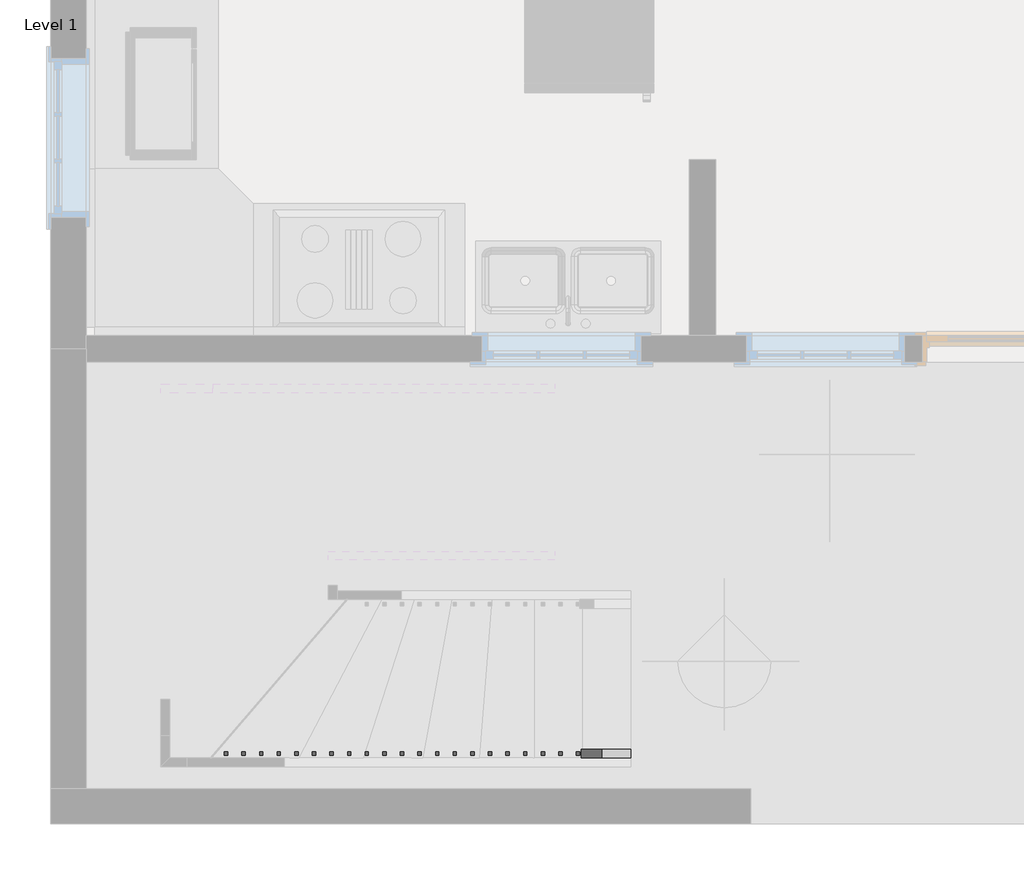
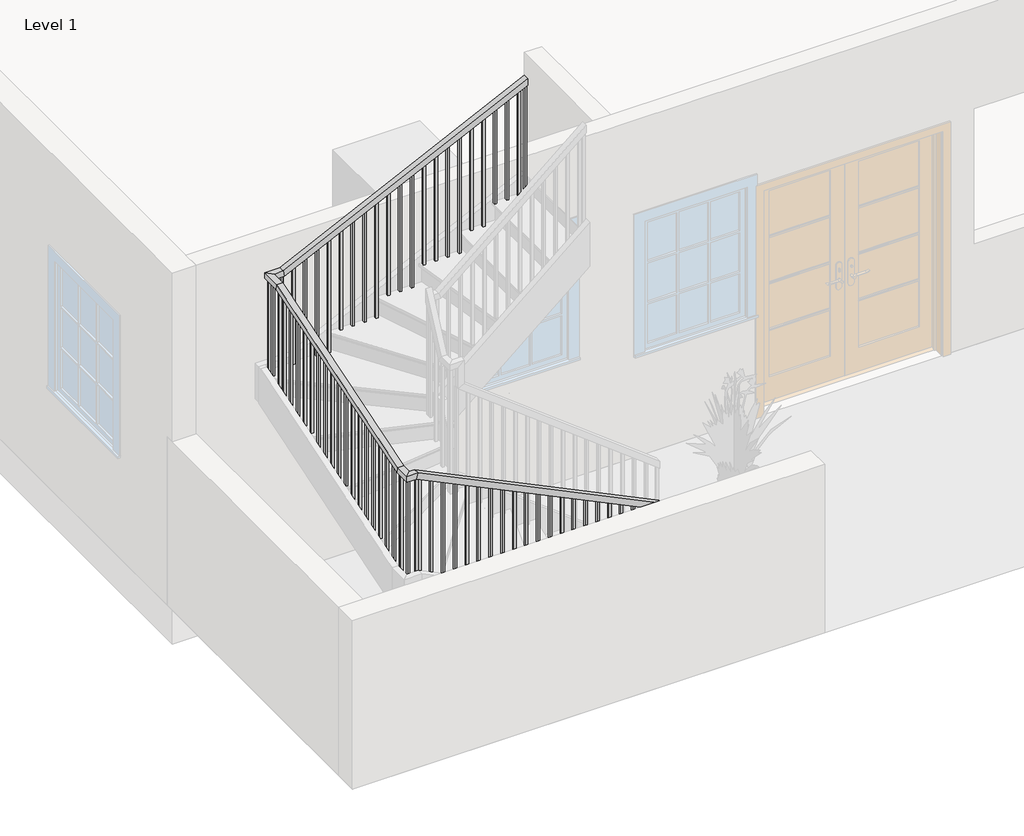
# One storey, part 2 of 3: 1 railing.
"""IFC4 building model written with IfcOpenShell, lengths in millimetres."""

from ifc_helpers import new_model, si_unit, frame, origin, place, context, project, spatial, polyline, outline, extrude, faceted_brep, element, save

model = new_model("IFC4")

# Units and contexts
model_context = context("Model", 3, world=origin())
ifc_project = project(units=[si_unit("LENGTHUNIT", "METRE", prefix="MILLI")], contexts=[model_context])

# Site, building, storey
site = spatial("IfcSite", under=ifc_project)
building = spatial("IfcBuilding", under=site)
storey = spatial("IfcBuildingStorey", under=building, Name="Level 1", Elevation=0.0)

# Railing
placement = place(None, origin())
element("IfcRailing", 1, ObjectType="Handrail - Rectangular", at=placement, inside=storey, context=model_context, shape_type="SolidModel", body=[
    faceted_brep([(-8086.227471, 2208.1174997, 1118.3371319), (-8086.227471, 2208.1174997, 1061.9393688), (-8086.227471, 2258.9174997, 1061.9393688), (-8086.227471, 2258.9174997, 1118.3371319), (-10651.2149162, 2208.1174997, 2355.2002855), (-10662.8234698, 2208.1174997, 2304.4002855), (-10662.8234698, 2258.9174997, 2304.4002855), (-10651.2149162, 2258.9174997, 2355.2002855), (-10747.2073372, 2208.1174997, 2355.2002855), (-10747.2073372, 2208.1174997, 2304.4002855), (-10696.4073372, 2258.9174997, 2304.4002855), (-10696.4073372, 2258.9174997, 2355.2002855), (-10747.2073372, 2341.0593041, 2355.2002855), (-10747.2073372, 2348.9073224, 2304.4002855), (-10696.4073372, 2348.9073224, 2304.4002855), (-10696.4073372, 2341.0593041, 2355.2002855), (-10747.2073372, 4134.1159277, 2922.7594886), (-10747.2073372, 4141.963946, 2871.9594886), (-10696.4073372, 4141.963946, 2871.9594886), (-10696.4073372, 4134.1159277, 2922.7594886), (-10747.2073372, 4316.3174997, 2922.7594886), (-10747.2073372, 4316.3174997, 2871.9594886), (-10696.4073372, 4265.5174997, 2871.9594886), (-10696.4073372, 4265.5174997, 2922.7594886), (-10618.3172645, 4316.3174997, 2922.7594886), (-10606.7656022, 4316.3174997, 2871.9594886), (-10606.7656022, 4265.5174997, 2871.9594886), (-10618.3172645, 4265.5174997, 2922.7594886), (-8524.2221093, 4316.3174997, 3927.0637322), (-8524.2221093, 4265.5174997, 3927.0637322), (-8524.2221093, 4265.5174997, 3870.7236862), (-8524.2221093, 4316.3174997, 3870.7236862)], [[[0, 1, 2, 3]], [[1, 0, 4, 5]], [[2, 1, 5, 6]], [[3, 2, 6, 7]], [[0, 3, 7, 4]], [[5, 4, 8, 9]], [[6, 5, 9, 10]], [[7, 6, 10, 11]], [[4, 7, 11, 8]], [[9, 8, 12, 13]], [[10, 9, 13, 14]], [[11, 10, 14, 15]], [[8, 11, 15, 12]], [[13, 12, 16, 17]], [[14, 13, 17, 18]], [[15, 14, 18, 19]], [[12, 15, 19, 16]], [[17, 16, 20, 21]], [[18, 17, 21, 22]], [[19, 18, 22, 23]], [[16, 19, 23, 20]], [[21, 20, 24, 25]], [[22, 21, 25, 26]], [[23, 22, 26, 27]], [[20, 23, 27, 24]], [[28, 29, 30, 31]], [[25, 24, 28, 31]], [[26, 25, 31, 30]], [[27, 26, 30, 29]], [[24, 27, 29, 28]]]),
    extrude(outline(polyline([(3836.3754735, -8595.8422645), (2878.6666667, -8595.8422645), (2878.6666667, -8576.7922645), (3845.5116371, -8576.7922645), (3836.3754735, -8595.8422645)])), frame((0.0, 4281.3924997, 0.0), z_axis=(0.0, 1.0, 0.0), x_axis=(0.0, 0.0, 1.0)), (0.0, 0.0, 1.0), 19.05),
    extrude(outline(polyline([(3787.6492679, -8697.4422645), (2878.6666667, -8697.4422645), (2878.6666667, -8678.3922645), (3796.7854315, -8678.3922645), (3787.6492679, -8697.4422645)])), frame((0.0, 4281.3924997, 0.0), z_axis=(0.0, 1.0, 0.0), x_axis=(0.0, 0.0, 1.0)), (0.0, 0.0, 1.0), 19.05),
    extrude(outline(polyline([(3738.9230623, -8799.0422645), (2878.6666667, -8799.0422645), (2878.6666667, -8779.9922645), (3748.0592258, -8779.9922645), (3738.9230623, -8799.0422645)])), frame((0.0, 4281.3924997, 0.0), z_axis=(0.0, 1.0, 0.0), x_axis=(0.0, 0.0, 1.0)), (0.0, 0.0, 1.0), 19.05),
    extrude(outline(polyline([(3690.1968566, -8900.6422645), (2709.3333333, -8900.6422645), (2709.3333333, -8881.5922645), (3699.3330202, -8881.5922645), (3690.1968566, -8900.6422645)])), frame((0.0, 4281.3924997, 0.0), z_axis=(0.0, 1.0, 0.0), x_axis=(0.0, 0.0, 1.0)), (0.0, 0.0, 1.0), 19.05),
    extrude(outline(polyline([(3641.470651, -9002.2422645), (2709.3333333, -9002.2422645), (2709.3333333, -8983.1922645), (3650.6068146, -8983.1922645), (3641.470651, -9002.2422645)])), frame((0.0, 4281.3924997, 0.0), z_axis=(0.0, 1.0, 0.0), x_axis=(0.0, 0.0, 1.0)), (0.0, 0.0, 1.0), 19.05),
    extrude(outline(polyline([(3592.7444454, -9103.8422645), (2540.0, -9103.8422645), (2540.0, -9084.7922645), (3601.8806089, -9084.7922645), (3592.7444454, -9103.8422645)])), frame((0.0, 4281.3924997, 0.0), z_axis=(0.0, 1.0, 0.0), x_axis=(0.0, 0.0, 1.0)), (0.0, 0.0, 1.0), 19.05),
    extrude(outline(polyline([(3544.0182397, -9205.4422645), (2540.0, -9205.4422645), (2540.0, -9186.3922645), (3553.1544033, -9186.3922645), (3544.0182397, -9205.4422645)])), frame((0.0, 4281.3924997, 0.0), z_axis=(0.0, 1.0, 0.0), x_axis=(0.0, 0.0, 1.0)), (0.0, 0.0, 1.0), 19.05),
    extrude(outline(polyline([(3495.2920341, -9307.0422645), (2540.0, -9307.0422645), (2540.0, -9287.9922645), (3504.4281977, -9287.9922645), (3495.2920341, -9307.0422645)])), frame((0.0, 4281.3924997, 0.0), z_axis=(0.0, 1.0, 0.0), x_axis=(0.0, 0.0, 1.0)), (0.0, 0.0, 1.0), 19.05),
    extrude(outline(polyline([(3446.5658285, -9408.6422645), (2540.0, -9408.6422645), (2540.0, -9389.5922645), (3455.701992, -9389.5922645), (3446.5658285, -9408.6422645)])), frame((0.0, 4281.3924997, 0.0), z_axis=(0.0, 1.0, 0.0), x_axis=(0.0, 0.0, 1.0)), (0.0, 0.0, 1.0), 19.05),
    extrude(outline(polyline([(3397.8396228, -9510.2422645), (2370.6666667, -9510.2422645), (2370.6666667, -9491.1922645), (3406.9757864, -9491.1922645), (3397.8396228, -9510.2422645)])), frame((0.0, 4281.3924997, 0.0), z_axis=(0.0, 1.0, 0.0), x_axis=(0.0, 0.0, 1.0)), (0.0, 0.0, 1.0), 19.05),
    extrude(outline(polyline([(3349.1134172, -9611.8422645), (2370.6666667, -9611.8422645), (2370.6666667, -9592.7922645), (3358.2495808, -9592.7922645), (3349.1134172, -9611.8422645)])), frame((0.0, 4281.3924997, 0.0), z_axis=(0.0, 1.0, 0.0), x_axis=(0.0, 0.0, 1.0)), (0.0, 0.0, 1.0), 19.05),
    extrude(outline(polyline([(3300.3872116, -9713.4422645), (2370.6666667, -9713.4422645), (2370.6666667, -9694.3922645), (3309.5233751, -9694.3922645), (3300.3872116, -9713.4422645)])), frame((0.0, 4281.3924997, 0.0), z_axis=(0.0, 1.0, 0.0), x_axis=(0.0, 0.0, 1.0)), (0.0, 0.0, 1.0), 19.05),
    extrude(outline(polyline([(3251.6610059, -9815.0422645), (2201.3333333, -9815.0422645), (2201.3333333, -9795.9922645), (3260.7971695, -9795.9922645), (3251.6610059, -9815.0422645)])), frame((0.0, 4281.3924997, 0.0), z_axis=(0.0, 1.0, 0.0), x_axis=(0.0, 0.0, 1.0)), (0.0, 0.0, 1.0), 19.05),
    extrude(outline(polyline([(3202.9348003, -9916.6422645), (2201.3333333, -9916.6422645), (2201.3333333, -9897.5922645), (3212.0709639, -9897.5922645), (3202.9348003, -9916.6422645)])), frame((0.0, 4281.3924997, 0.0), z_axis=(0.0, 1.0, 0.0), x_axis=(0.0, 0.0, 1.0)), (0.0, 0.0, 1.0), 19.05),
    extrude(outline(polyline([(3154.2085947, -10018.2422645), (2201.3333333, -10018.2422645), (2201.3333333, -9999.1922645), (3163.3447582, -9999.1922645), (3154.2085947, -10018.2422645)])), frame((0.0, 4281.3924997, 0.0), z_axis=(0.0, 1.0, 0.0), x_axis=(0.0, 0.0, 1.0)), (0.0, 0.0, 1.0), 19.05),
    extrude(outline(polyline([(3105.482389, -10119.8422645), (2201.3333333, -10119.8422645), (2201.3333333, -10100.7922645), (3114.6185526, -10100.7922645), (3105.482389, -10119.8422645)])), frame((0.0, 4281.3924997, 0.0), z_axis=(0.0, 1.0, 0.0), x_axis=(0.0, 0.0, 1.0)), (0.0, 0.0, 1.0), 19.05),
    extrude(outline(polyline([(3056.7561834, -10221.4422645), (2032.0, -10221.4422645), (2032.0, -10202.3922645), (3065.892347, -10202.3922645), (3056.7561834, -10221.4422645)])), frame((0.0, 4281.3924997, 0.0), z_axis=(0.0, 1.0, 0.0), x_axis=(0.0, 0.0, 1.0)), (0.0, 0.0, 1.0), 19.05),
    extrude(outline(polyline([(3008.0299778, -10323.0422645), (2032.0, -10323.0422645), (2032.0, -10303.9922645), (3017.1661413, -10303.9922645), (3008.0299778, -10323.0422645)])), frame((0.0, 4281.3924997, 0.0), z_axis=(0.0, 1.0, 0.0), x_axis=(0.0, 0.0, 1.0)), (0.0, 0.0, 1.0), 19.05),
    extrude(outline(polyline([(2959.3037721, -10424.6422645), (2032.0, -10424.6422645), (2032.0, -10405.5922645), (2968.4399357, -10405.5922645), (2959.3037721, -10424.6422645)])), frame((0.0, 4281.3924997, 0.0), z_axis=(0.0, 1.0, 0.0), x_axis=(0.0, 0.0, 1.0)), (0.0, 0.0, 1.0), 19.05),
    extrude(outline(polyline([(2910.5010439, -10526.2422645), (2032.0, -10526.2422645), (2032.0, -10507.1922645), (2919.6871485, -10507.1922645), (2910.5010439, -10526.2422645)])), frame((0.0, 4281.3924997, 0.0), z_axis=(0.0, 1.0, 0.0), x_axis=(0.0, 0.0, 1.0)), (0.0, 0.0, 1.0), 19.05),
    extrude(outline(polyline([(-10629.7323372, 4300.4424997), (-10610.6823372, 4300.4424997), (-10610.6823372, 4281.3924997), (-10629.7323372, 4281.3924997), (-10629.7323372, 4300.4424997)])), frame((0.0, 0.0, 2032.0), z_axis=(0.0, 0.0, 1.0), x_axis=(1.0, 0.0, 0.0)), (0.0, 0.0, 1.0), 839.9594886),
    extrude(outline(polyline([(-10731.3323372, 4226.1909277), (-10731.3323372, 4245.2409277), (-10712.2823372, 4245.2409277), (-10712.2823372, 4226.1909277), (-10731.3323372, 4226.1909277)])), frame((0.0, 0.0, 2032.0), z_axis=(0.0, 0.0, 1.0), x_axis=(1.0, 0.0, 0.0)), (0.0, 0.0, 1.0), 839.9594886),
    extrude(outline(polyline([(4077.7843041, 2851.6445995), (4077.7843041, 1862.6666667), (4058.7343041, 1862.6666667), (4058.7343041, 2845.6146713), (4077.7843041, 2851.6445995)])), frame((-10731.3323372, 0.0, 0.0), z_axis=(1.0, 0.0, 0.0), x_axis=(0.0, 1.0, 0.0)), (0.0, 0.0, 1.0), 19.05),
    extrude(outline(polyline([(3976.1843041, 2819.4849821), (3976.1843041, 1862.6666667), (3957.1343041, 1862.6666667), (3957.1343041, 2813.4550538), (3976.1843041, 2819.4849821)])), frame((-10731.3323372, 0.0, 0.0), z_axis=(1.0, 0.0, 0.0), x_axis=(0.0, 1.0, 0.0)), (0.0, 0.0, 1.0), 19.05),
    extrude(outline(polyline([(3874.5843041, 2787.3253647), (3874.5843041, 1862.6666667), (3855.5343041, 1862.6666667), (3855.5343041, 2781.2954364), (3874.5843041, 2787.3253647)])), frame((-10731.3323372, 0.0, 0.0), z_axis=(1.0, 0.0, 0.0), x_axis=(0.0, 1.0, 0.0)), (0.0, 0.0, 1.0), 19.05),
    extrude(outline(polyline([(3772.9843041, 2755.1657473), (3772.9843041, 1862.6666667), (3753.9343041, 1862.6666667), (3753.9343041, 2749.135819), (3772.9843041, 2755.1657473)])), frame((-10731.3323372, 0.0, 0.0), z_axis=(1.0, 0.0, 0.0), x_axis=(0.0, 1.0, 0.0)), (0.0, 0.0, 1.0), 19.05),
    extrude(outline(polyline([(3671.3843041, 2723.0061298), (3671.3843041, 1862.6666667), (3652.3343041, 1862.6666667), (3652.3343041, 2716.9762016), (3671.3843041, 2723.0061298)])), frame((-10731.3323372, 0.0, 0.0), z_axis=(1.0, 0.0, 0.0), x_axis=(0.0, 1.0, 0.0)), (0.0, 0.0, 1.0), 19.05),
    extrude(outline(polyline([(3569.7843041, 2690.8465124), (3569.7843041, 1693.3333333), (3550.7343041, 1693.3333333), (3550.7343041, 2684.8165841), (3569.7843041, 2690.8465124)])), frame((-10731.3323372, 0.0, 0.0), z_axis=(1.0, 0.0, 0.0), x_axis=(0.0, 1.0, 0.0)), (0.0, 0.0, 1.0), 19.05),
    extrude(outline(polyline([(3468.1843041, 2658.686895), (3468.1843041, 1693.3333333), (3449.1343041, 1693.3333333), (3449.1343041, 2652.6569667), (3468.1843041, 2658.686895)])), frame((-10731.3323372, 0.0, 0.0), z_axis=(1.0, 0.0, 0.0), x_axis=(0.0, 1.0, 0.0)), (0.0, 0.0, 1.0), 19.05),
    extrude(outline(polyline([(3366.5843041, 2626.5272776), (3366.5843041, 1693.3333333), (3347.5343041, 1693.3333333), (3347.5343041, 2620.4973493), (3366.5843041, 2626.5272776)])), frame((-10731.3323372, 0.0, 0.0), z_axis=(1.0, 0.0, 0.0), x_axis=(0.0, 1.0, 0.0)), (0.0, 0.0, 1.0), 19.05),
    extrude(outline(polyline([(3264.9843041, 2594.3676601), (3264.9843041, 1693.3333333), (3245.9343041, 1693.3333333), (3245.9343041, 2588.3377319), (3264.9843041, 2594.3676601)])), frame((-10731.3323372, 0.0, 0.0), z_axis=(1.0, 0.0, 0.0), x_axis=(0.0, 1.0, 0.0)), (0.0, 0.0, 1.0), 19.05),
    extrude(outline(polyline([(3163.3843041, 2562.2080427), (3163.3843041, 1693.3333333), (3144.3343041, 1693.3333333), (3144.3343041, 2556.1781144), (3163.3843041, 2562.2080427)])), frame((-10731.3323372, 0.0, 0.0), z_axis=(1.0, 0.0, 0.0), x_axis=(0.0, 1.0, 0.0)), (0.0, 0.0, 1.0), 19.05),
    extrude(outline(polyline([(3061.7843041, 2530.0484253), (3061.7843041, 1524.0), (3042.7343041, 1524.0), (3042.7343041, 2524.018497), (3061.7843041, 2530.0484253)])), frame((-10731.3323372, 0.0, 0.0), z_axis=(1.0, 0.0, 0.0), x_axis=(0.0, 1.0, 0.0)), (0.0, 0.0, 1.0), 19.05),
    extrude(outline(polyline([(2960.1843041, 2497.8888078), (2960.1843041, 1524.0), (2941.1343041, 1524.0), (2941.1343041, 2491.8588796), (2960.1843041, 2497.8888078)])), frame((-10731.3323372, 0.0, 0.0), z_axis=(1.0, 0.0, 0.0), x_axis=(0.0, 1.0, 0.0)), (0.0, 0.0, 1.0), 19.05),
    extrude(outline(polyline([(2858.5843041, 2465.7291904), (2858.5843041, 1524.0), (2839.5343041, 1524.0), (2839.5343041, 2459.6992621), (2858.5843041, 2465.7291904)])), frame((-10731.3323372, 0.0, 0.0), z_axis=(1.0, 0.0, 0.0), x_axis=(0.0, 1.0, 0.0)), (0.0, 0.0, 1.0), 19.05),
    extrude(outline(polyline([(2756.9843041, 2433.569573), (2756.9843041, 1524.0), (2737.9343041, 1524.0), (2737.9343041, 2427.5396447), (2756.9843041, 2433.569573)])), frame((-10731.3323372, 0.0, 0.0), z_axis=(1.0, 0.0, 0.0), x_axis=(0.0, 1.0, 0.0)), (0.0, 0.0, 1.0), 19.05),
    extrude(outline(polyline([(2655.3843041, 2401.4099556), (2655.3843041, 1524.0), (2636.3343041, 1524.0), (2636.3343041, 2395.3800273), (2655.3843041, 2401.4099556)])), frame((-10731.3323372, 0.0, 0.0), z_axis=(1.0, 0.0, 0.0), x_axis=(0.0, 1.0, 0.0)), (0.0, 0.0, 1.0), 19.05),
    extrude(outline(polyline([(2553.7843041, 2369.2503381), (2553.7843041, 1354.6666667), (2534.7343041, 1354.6666667), (2534.7343041, 2363.2204099), (2553.7843041, 2369.2503381)])), frame((-10731.3323372, 0.0, 0.0), z_axis=(1.0, 0.0, 0.0), x_axis=(0.0, 1.0, 0.0)), (0.0, 0.0, 1.0), 19.05),
    extrude(outline(polyline([(2452.1843041, 2337.0907207), (2452.1843041, 1354.6666667), (2433.1343041, 1354.6666667), (2433.1343041, 2331.0607924), (2452.1843041, 2337.0907207)])), frame((-10731.3323372, 0.0, 0.0), z_axis=(1.0, 0.0, 0.0), x_axis=(0.0, 1.0, 0.0)), (0.0, 0.0, 1.0), 19.05),
    extrude(outline(polyline([(-10731.3323372, 2325.5924997), (-10731.3323372, 2344.6424997), (-10712.2823372, 2344.6424997), (-10712.2823372, 2325.5924997), (-10731.3323372, 2325.5924997)])), frame((0.0, 0.0, 1354.6666667), z_axis=(0.0, 0.0, 1.0), x_axis=(1.0, 0.0, 0.0)), (0.0, 0.0, 1.0), 949.7336188),
    extrude(outline(polyline([(2291.3463733, -10635.752471), (1354.6666667, -10635.752471), (1354.6666667, -10616.702471), (2282.1602686, -10616.702471), (2291.3463733, -10635.752471)])), frame((0.0, 2223.9924997, 0.0), z_axis=(0.0, 1.0, 0.0), x_axis=(0.0, 0.0, 1.0)), (0.0, 0.0, 1.0), 19.05),
    extrude(outline(polyline([(2242.3538152, -10534.152471), (1354.6666667, -10534.152471), (1354.6666667, -10515.102471), (2233.1677105, -10515.102471), (2242.3538152, -10534.152471)])), frame((0.0, 2223.9924997, 0.0), z_axis=(0.0, 1.0, 0.0), x_axis=(0.0, 0.0, 1.0)), (0.0, 0.0, 1.0), 19.05),
    extrude(outline(polyline([(2193.3612571, -10432.552471), (1185.3333333, -10432.552471), (1185.3333333, -10413.502471), (2184.1751524, -10413.502471), (2193.3612571, -10432.552471)])), frame((0.0, 2223.9924997, 0.0), z_axis=(0.0, 1.0, 0.0), x_axis=(0.0, 0.0, 1.0)), (0.0, 0.0, 1.0), 19.05),
    extrude(outline(polyline([(2144.368699, -10330.952471), (1185.3333333, -10330.952471), (1185.3333333, -10311.902471), (2135.1825944, -10311.902471), (2144.368699, -10330.952471)])), frame((0.0, 2223.9924997, 0.0), z_axis=(0.0, 1.0, 0.0), x_axis=(0.0, 0.0, 1.0)), (0.0, 0.0, 1.0), 19.05),
    extrude(outline(polyline([(2095.3761409, -10229.352471), (1185.3333333, -10229.352471), (1185.3333333, -10210.302471), (2086.1900363, -10210.302471), (2095.3761409, -10229.352471)])), frame((0.0, 2223.9924997, 0.0), z_axis=(0.0, 1.0, 0.0), x_axis=(0.0, 0.0, 1.0)), (0.0, 0.0, 1.0), 19.05),
    extrude(outline(polyline([(2046.3835828, -10127.752471), (1185.3333333, -10127.752471), (1185.3333333, -10108.702471), (2037.1974782, -10108.702471), (2046.3835828, -10127.752471)])), frame((0.0, 2223.9924997, 0.0), z_axis=(0.0, 1.0, 0.0), x_axis=(0.0, 0.0, 1.0)), (0.0, 0.0, 1.0), 19.05),
    extrude(outline(polyline([(1997.3910247, -10026.152471), (1185.3333333, -10026.152471), (1185.3333333, -10007.102471), (1988.2049201, -10007.102471), (1997.3910247, -10026.152471)])), frame((0.0, 2223.9924997, 0.0), z_axis=(0.0, 1.0, 0.0), x_axis=(0.0, 0.0, 1.0)), (0.0, 0.0, 1.0), 19.05),
    extrude(outline(polyline([(1948.3984667, -9924.552471), (1016.0, -9924.552471), (1016.0, -9905.502471), (1939.212362, -9905.502471), (1948.3984667, -9924.552471)])), frame((0.0, 2223.9924997, 0.0), z_axis=(0.0, 1.0, 0.0), x_axis=(0.0, 0.0, 1.0)), (0.0, 0.0, 1.0), 19.05),
    extrude(outline(polyline([(1899.4059086, -9822.952471), (1016.0, -9822.952471), (1016.0, -9803.902471), (1890.2198039, -9803.902471), (1899.4059086, -9822.952471)])), frame((0.0, 2223.9924997, 0.0), z_axis=(0.0, 1.0, 0.0), x_axis=(0.0, 0.0, 1.0)), (0.0, 0.0, 1.0), 19.05),
    extrude(outline(polyline([(1850.4133505, -9721.352471), (1016.0, -9721.352471), (1016.0, -9702.302471), (1841.2272458, -9702.302471), (1850.4133505, -9721.352471)])), frame((0.0, 2223.9924997, 0.0), z_axis=(0.0, 1.0, 0.0), x_axis=(0.0, 0.0, 1.0)), (0.0, 0.0, 1.0), 19.05),
    extrude(outline(polyline([(1801.4207924, -9619.752471), (846.6666667, -9619.752471), (846.6666667, -9600.702471), (1792.2346878, -9600.702471), (1801.4207924, -9619.752471)])), frame((0.0, 2223.9924997, 0.0), z_axis=(0.0, 1.0, 0.0), x_axis=(0.0, 0.0, 1.0)), (0.0, 0.0, 1.0), 19.05),
    extrude(outline(polyline([(1752.4282343, -9518.152471), (846.6666667, -9518.152471), (846.6666667, -9499.102471), (1743.2421297, -9499.102471), (1752.4282343, -9518.152471)])), frame((0.0, 2223.9924997, 0.0), z_axis=(0.0, 1.0, 0.0), x_axis=(0.0, 0.0, 1.0)), (0.0, 0.0, 1.0), 19.05),
    extrude(outline(polyline([(1703.4356762, -9416.552471), (846.6666667, -9416.552471), (846.6666667, -9397.502471), (1694.2495716, -9397.502471), (1703.4356762, -9416.552471)])), frame((0.0, 2223.9924997, 0.0), z_axis=(0.0, 1.0, 0.0), x_axis=(0.0, 0.0, 1.0)), (0.0, 0.0, 1.0), 19.05),
    extrude(outline(polyline([(1654.4431181, -9314.952471), (846.6666667, -9314.952471), (846.6666667, -9295.902471), (1645.2570135, -9295.902471), (1654.4431181, -9314.952471)])), frame((0.0, 2223.9924997, 0.0), z_axis=(0.0, 1.0, 0.0), x_axis=(0.0, 0.0, 1.0)), (0.0, 0.0, 1.0), 19.05),
    extrude(outline(polyline([(1605.4505601, -9213.352471), (677.3333333, -9213.352471), (677.3333333, -9194.302471), (1596.2644554, -9194.302471), (1605.4505601, -9213.352471)])), frame((0.0, 2223.9924997, 0.0), z_axis=(0.0, 1.0, 0.0), x_axis=(0.0, 0.0, 1.0)), (0.0, 0.0, 1.0), 19.05),
    extrude(outline(polyline([(1556.458002, -9111.752471), (677.3333333, -9111.752471), (677.3333333, -9092.702471), (1547.2718973, -9092.702471), (1556.458002, -9111.752471)])), frame((0.0, 2223.9924997, 0.0), z_axis=(0.0, 1.0, 0.0), x_axis=(0.0, 0.0, 1.0)), (0.0, 0.0, 1.0), 19.05),
    extrude(outline(polyline([(1507.4654439, -9010.152471), (677.3333333, -9010.152471), (677.3333333, -8991.102471), (1498.2793392, -8991.102471), (1507.4654439, -9010.152471)])), frame((0.0, 2223.9924997, 0.0), z_axis=(0.0, 1.0, 0.0), x_axis=(0.0, 0.0, 1.0)), (0.0, 0.0, 1.0), 19.05),
    extrude(outline(polyline([(1458.4728858, -8908.552471), (508.0, -8908.552471), (508.0, -8889.502471), (1449.2867812, -8889.502471), (1458.4728858, -8908.552471)])), frame((0.0, 2223.9924997, 0.0), z_axis=(0.0, 1.0, 0.0), x_axis=(0.0, 0.0, 1.0)), (0.0, 0.0, 1.0), 19.05),
    extrude(outline(polyline([(1409.4803277, -8806.952471), (508.0, -8806.952471), (508.0, -8787.902471), (1400.2942231, -8787.902471), (1409.4803277, -8806.952471)])), frame((0.0, 2223.9924997, 0.0), z_axis=(0.0, 1.0, 0.0), x_axis=(0.0, 0.0, 1.0)), (0.0, 0.0, 1.0), 19.05),
    extrude(outline(polyline([(1360.4877696, -8705.352471), (508.0, -8705.352471), (508.0, -8686.302471), (1351.301665, -8686.302471), (1360.4877696, -8705.352471)])), frame((0.0, 2223.9924997, 0.0), z_axis=(0.0, 1.0, 0.0), x_axis=(0.0, 0.0, 1.0)), (0.0, 0.0, 1.0), 19.05),
    extrude(outline(polyline([(1311.4952115, -8603.752471), (338.6666667, -8603.752471), (338.6666667, -8584.702471), (1302.3091069, -8584.702471), (1311.4952115, -8603.752471)])), frame((0.0, 2223.9924997, 0.0), z_axis=(0.0, 1.0, 0.0), x_axis=(0.0, 0.0, 1.0)), (0.0, 0.0, 1.0), 19.05),
    extrude(outline(polyline([(1262.5026535, -8502.152471), (338.6666667, -8502.152471), (338.6666667, -8483.102471), (1253.3165488, -8483.102471), (1262.5026535, -8502.152471)])), frame((0.0, 2223.9924997, 0.0), z_axis=(0.0, 1.0, 0.0), x_axis=(0.0, 0.0, 1.0)), (0.0, 0.0, 1.0), 19.05),
    extrude(outline(polyline([(1213.5100954, -8400.552471), (338.6666667, -8400.552471), (338.6666667, -8381.502471), (1204.3239907, -8381.502471), (1213.5100954, -8400.552471)])), frame((0.0, 2223.9924997, 0.0), z_axis=(0.0, 1.0, 0.0), x_axis=(0.0, 0.0, 1.0)), (0.0, 0.0, 1.0), 19.05),
    extrude(outline(polyline([(1164.5175373, -8298.952471), (169.3333333, -8298.952471), (169.3333333, -8279.902471), (1155.3314326, -8279.902471), (1164.5175373, -8298.952471)])), frame((0.0, 2223.9924997, 0.0), z_axis=(0.0, 1.0, 0.0), x_axis=(0.0, 0.0, 1.0)), (0.0, 0.0, 1.0), 19.05),
    extrude(outline(polyline([(1115.5249792, -8197.352471), (169.3333333, -8197.352471), (169.3333333, -8178.302471), (1106.3388746, -8178.302471), (1115.5249792, -8197.352471)])), frame((0.0, 2223.9924997, 0.0), z_axis=(0.0, 1.0, 0.0), x_axis=(0.0, 0.0, 1.0)), (0.0, 0.0, 1.0), 19.05),
    extrude(outline(polyline([(-10627.8422645, 4300.4424997), (-10608.7922645, 4300.4424997), (-10608.7922645, 4281.3924997), (-10627.8422645, 4281.3924997), (-10627.8422645, 4300.4424997)])), frame((0.0, 0.0, 2032.0), z_axis=(0.0, 0.0, 1.0), x_axis=(1.0, 0.0, 0.0)), (0.0, 0.0, 1.0), 839.9594886),
    extrude(outline(polyline([(-10731.3323372, 4281.3924997), (-10731.3323372, 4300.4424997), (-10712.2823372, 4300.4424997), (-10712.2823372, 4281.3924997), (-10731.3323372, 4281.3924997)])), frame((0.0, 0.0, 2032.0), z_axis=(0.0, 0.0, 1.0), x_axis=(1.0, 0.0, 0.0)), (0.0, 0.0, 1.0), 839.9594886),
    extrude(outline(polyline([(4143.6409277, 2872.4903064), (4143.6409277, 1862.6666667), (4124.5909277, 1862.6666667), (4124.5909277, 2866.4603782), (4143.6409277, 2872.4903064)])), frame((-10731.3323372, 0.0, 0.0), z_axis=(1.0, 0.0, 0.0), x_axis=(0.0, 1.0, 0.0)), (0.0, 0.0, 1.0), 19.05),
    extrude(outline(polyline([(-10731.3323372, 2331.5343041), (-10731.3323372, 2350.5843041), (-10712.2823372, 2350.5843041), (-10712.2823372, 2331.5343041), (-10731.3323372, 2331.5343041)])), frame((0.0, 0.0, 1354.6666667), z_axis=(0.0, 0.0, 1.0), x_axis=(1.0, 0.0, 0.0)), (0.0, 0.0, 1.0), 949.7336188),
    extrude(outline(polyline([(-10712.2823372, 2223.9924997), (-10731.3323372, 2223.9924997), (-10731.3323372, 2243.0424997), (-10712.2823372, 2243.0424997), (-10712.2823372, 2223.9924997)])), frame((0.0, 0.0, 1354.6666667), z_axis=(0.0, 0.0, 1.0), x_axis=(1.0, 0.0, 0.0)), (0.0, 0.0, 1.0), 949.7336188),
    extrude(outline(polyline([(2303.3955746, -10660.7399162), (1354.6666667, -10660.7399162), (1354.6666667, -10641.6899162), (2294.20947, -10641.6899162), (2303.3955746, -10660.7399162)])), frame((0.0, 2223.9924997, 0.0), z_axis=(0.0, 1.0, 0.0), x_axis=(0.0, 0.0, 1.0)), (0.0, 0.0, 1.0), 19.05),
    extrude(outline(polyline([(3861.5875226, -8543.2721093), (2878.6666667, -8543.2721093), (2878.6666667, -8524.2221093), (3870.7236862, -8524.2221093), (3861.5875226, -8543.2721093)])), frame((0.0, 4281.3924997, 0.0), z_axis=(0.0, 1.0, 0.0), x_axis=(0.0, 0.0, 1.0)), (0.0, 0.0, 1.0), 19.05),
    extrude(outline(polyline([(1071.1254734, -8105.277471), (169.3333333, -8105.277471), (169.3333333, -8086.227471), (1061.9393688, -8086.227471), (1071.1254734, -8105.277471)])), frame((0.0, 2223.9924997, 0.0), z_axis=(0.0, 1.0, 0.0), x_axis=(0.0, 0.0, 1.0)), (0.0, 0.0, 1.0), 19.05),
])

save(model, "model.ifc")

# Revit data of these elements
# Type "Handrail - Rectangular"
#   Assembly Code = "C2010400"
#   built-in parameter 1008612 = 0.0416667 (stored number, unit not read)
#   built-in parameter 1008611 = 0.0416667 (stored number, unit not read)
#   built-in parameter 1008609 = 0.333333 (stored number, unit not read)
#   built-in parameter 1008604 = 0.166667 (stored number, unit not read)
#   built-in parameter 1008603 = 0.166667 (stored number, unit not read)
#   Railing Height = 3' - 0"
#   built-in parameter 1008630 = 2
#   built-in parameter 1008610 = 2
#   built-in parameter 1008618 = Baluster - Square : 3/4"
# Element 1 (IfcRailing, "Handrail - Rectangular")
#   Phase Created = New Construction
